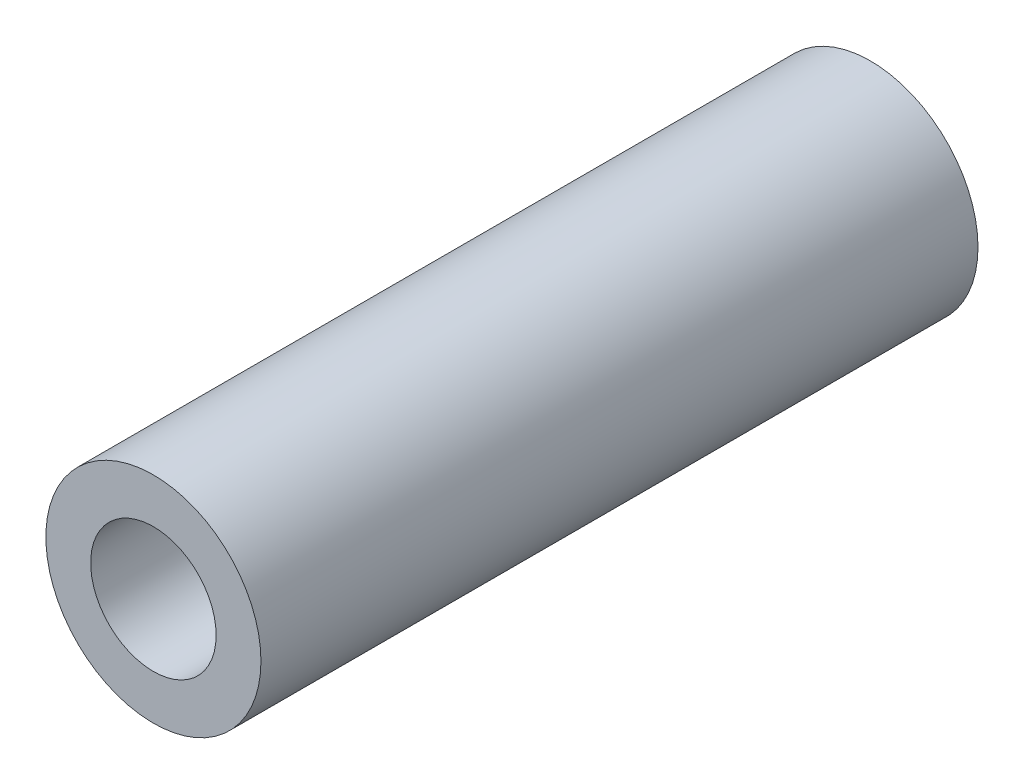
ISO-10303-21;
HEADER;
FILE_DESCRIPTION(('STEP AP214'),'2;1');
FILE_NAME('part.step','',(''),(''),'','','');
FILE_SCHEMA(('AUTOMOTIVE_DESIGN { 1 0 10303 214 1 1 1 1 }'));
ENDSEC;
DATA;
#1=APPLICATION_CONTEXT('core data for automotive mechanical design processes');
#2=APPLICATION_PROTOCOL_DEFINITION('international standard','automotive_design',2000,#1);
#3=PRODUCT_CONTEXT('',#1,'mechanical');
#4=PRODUCT('Part','Part','',(#3));
#5=PRODUCT_RELATED_PRODUCT_CATEGORY('part','',(#4));
#6=PRODUCT_DEFINITION_FORMATION('','',#4);
#7=PRODUCT_DEFINITION_CONTEXT('part definition',#1,'design');
#8=PRODUCT_DEFINITION('design','',#6,#7);
#9=PRODUCT_DEFINITION_SHAPE('','',#8);
#10=(LENGTH_UNIT() NAMED_UNIT(*) SI_UNIT(.MILLI.,.METRE.));
#11=(NAMED_UNIT(*) PLANE_ANGLE_UNIT() SI_UNIT($,.RADIAN.));
#12=(NAMED_UNIT(*) SI_UNIT($,.STERADIAN.) SOLID_ANGLE_UNIT());
#13=UNCERTAINTY_MEASURE_WITH_UNIT(LENGTH_MEASURE(1.E-05),#10,'distance_accuracy_value','');
#14=(GEOMETRIC_REPRESENTATION_CONTEXT(3) GLOBAL_UNCERTAINTY_ASSIGNED_CONTEXT((#13)) GLOBAL_UNIT_ASSIGNED_CONTEXT((#10,
#11,#12)) REPRESENTATION_CONTEXT('',''));
#15=CARTESIAN_POINT('',(0.,0.,0.));
#16=DIRECTION('',(0.,0.,1.));
#17=DIRECTION('',(1.,0.,0.));
#18=AXIS2_PLACEMENT_3D('',#15,#16,#17);
#19=CARTESIAN_POINT('',(0.,0.,10.));
#20=DIRECTION('',(0.,0.,1.));
#21=DIRECTION('',(1.,0.,0.));
#22=AXIS2_PLACEMENT_3D('',#19,#20,#21);
#23=PLANE('',#22);
#24=CARTESIAN_POINT('',(0.,0.,10.));
#25=DIRECTION('',(0.,0.,1.));
#26=DIRECTION('',(1.,0.,0.));
#27=AXIS2_PLACEMENT_3D('',#24,#25,#26);
#28=CIRCLE('',#27,3.);
#29=CARTESIAN_POINT('',(3.,0.,10.));
#30=VERTEX_POINT('',#29);
#31=EDGE_CURVE('E10',#30,#30,#28,.T.);
#32=ORIENTED_EDGE('',*,*,#31,.T.);
#33=EDGE_LOOP('',(#32));
#34=FACE_BOUND('',#33,.T.);
#35=CARTESIAN_POINT('',(0.,0.,10.));
#36=DIRECTION('',(0.,0.,1.));
#37=DIRECTION('',(1.,0.,0.));
#38=AXIS2_PLACEMENT_3D('',#35,#36,#37);
#39=CIRCLE('',#38,1.75);
#40=CARTESIAN_POINT('',(1.75,0.,10.));
#41=VERTEX_POINT('',#40);
#42=EDGE_CURVE('E48',#41,#41,#39,.T.);
#43=ORIENTED_EDGE('',*,*,#42,.F.);
#44=EDGE_LOOP('',(#43));
#45=FACE_BOUND('',#44,.T.);
#46=ADVANCED_FACE('F40',(#34,#45),#23,.T.);
#47=CARTESIAN_POINT('',(0.,0.,-10.));
#48=DIRECTION('',(0.,0.,1.));
#49=DIRECTION('',(1.,0.,0.));
#50=AXIS2_PLACEMENT_3D('',#47,#48,#49);
#51=PLANE('',#50);
#52=CARTESIAN_POINT('',(0.,0.,-10.));
#53=DIRECTION('',(0.,0.,1.));
#54=DIRECTION('',(1.,0.,0.));
#55=AXIS2_PLACEMENT_3D('',#52,#53,#54);
#56=CIRCLE('',#55,3.);
#57=CARTESIAN_POINT('',(3.,0.,-10.));
#58=VERTEX_POINT('',#57);
#59=EDGE_CURVE('E41',#58,#58,#56,.T.);
#60=ORIENTED_EDGE('',*,*,#59,.F.);
#61=EDGE_LOOP('',(#60));
#62=FACE_BOUND('',#61,.T.);
#63=CARTESIAN_POINT('',(0.,0.,-10.));
#64=DIRECTION('',(0.,0.,1.));
#65=DIRECTION('',(1.,0.,0.));
#66=AXIS2_PLACEMENT_3D('',#63,#64,#65);
#67=CIRCLE('',#66,1.75);
#68=CARTESIAN_POINT('',(1.75,0.,-10.));
#69=VERTEX_POINT('',#68);
#70=EDGE_CURVE('E49',#69,#69,#67,.T.);
#71=ORIENTED_EDGE('',*,*,#70,.T.);
#72=EDGE_LOOP('',(#71));
#73=FACE_BOUND('',#72,.T.);
#74=ADVANCED_FACE('F58',(#62,#73),#51,.F.);
#75=CARTESIAN_POINT('',(0.,0.,10.));
#76=DIRECTION('',(0.,0.,-1.));
#77=DIRECTION('',(-1.,0.,0.));
#78=AXIS2_PLACEMENT_3D('',#75,#76,#77);
#79=CYLINDRICAL_SURFACE('',#78,3.);
#80=ORIENTED_EDGE('',*,*,#31,.F.);
#81=EDGE_LOOP('',(#80));
#82=FACE_BOUND('',#81,.T.);
#83=ORIENTED_EDGE('',*,*,#59,.T.);
#84=EDGE_LOOP('',(#83));
#85=FACE_BOUND('',#84,.T.);
#86=ADVANCED_FACE('F39',(#82,#85),#79,.T.);
#87=CARTESIAN_POINT('',(0.,0.,10.));
#88=DIRECTION('',(0.,0.,-1.));
#89=DIRECTION('',(-1.,0.,0.));
#90=AXIS2_PLACEMENT_3D('',#87,#88,#89);
#91=CYLINDRICAL_SURFACE('',#90,1.75);
#92=ORIENTED_EDGE('',*,*,#42,.T.);
#93=EDGE_LOOP('',(#92));
#94=FACE_BOUND('',#93,.T.);
#95=ORIENTED_EDGE('',*,*,#70,.F.);
#96=EDGE_LOOP('',(#95));
#97=FACE_BOUND('',#96,.T.);
#98=ADVANCED_FACE('F57',(#94,#97),#91,.F.);
#99=CLOSED_SHELL('',(#46,#74,#86,#98));
#100=MANIFOLD_SOLID_BREP('B2',#99);
#101=ADVANCED_BREP_SHAPE_REPRESENTATION('',(#18,#100),#14);
#102=SHAPE_DEFINITION_REPRESENTATION(#9,#101);
ENDSEC;
END-ISO-10303-21;
